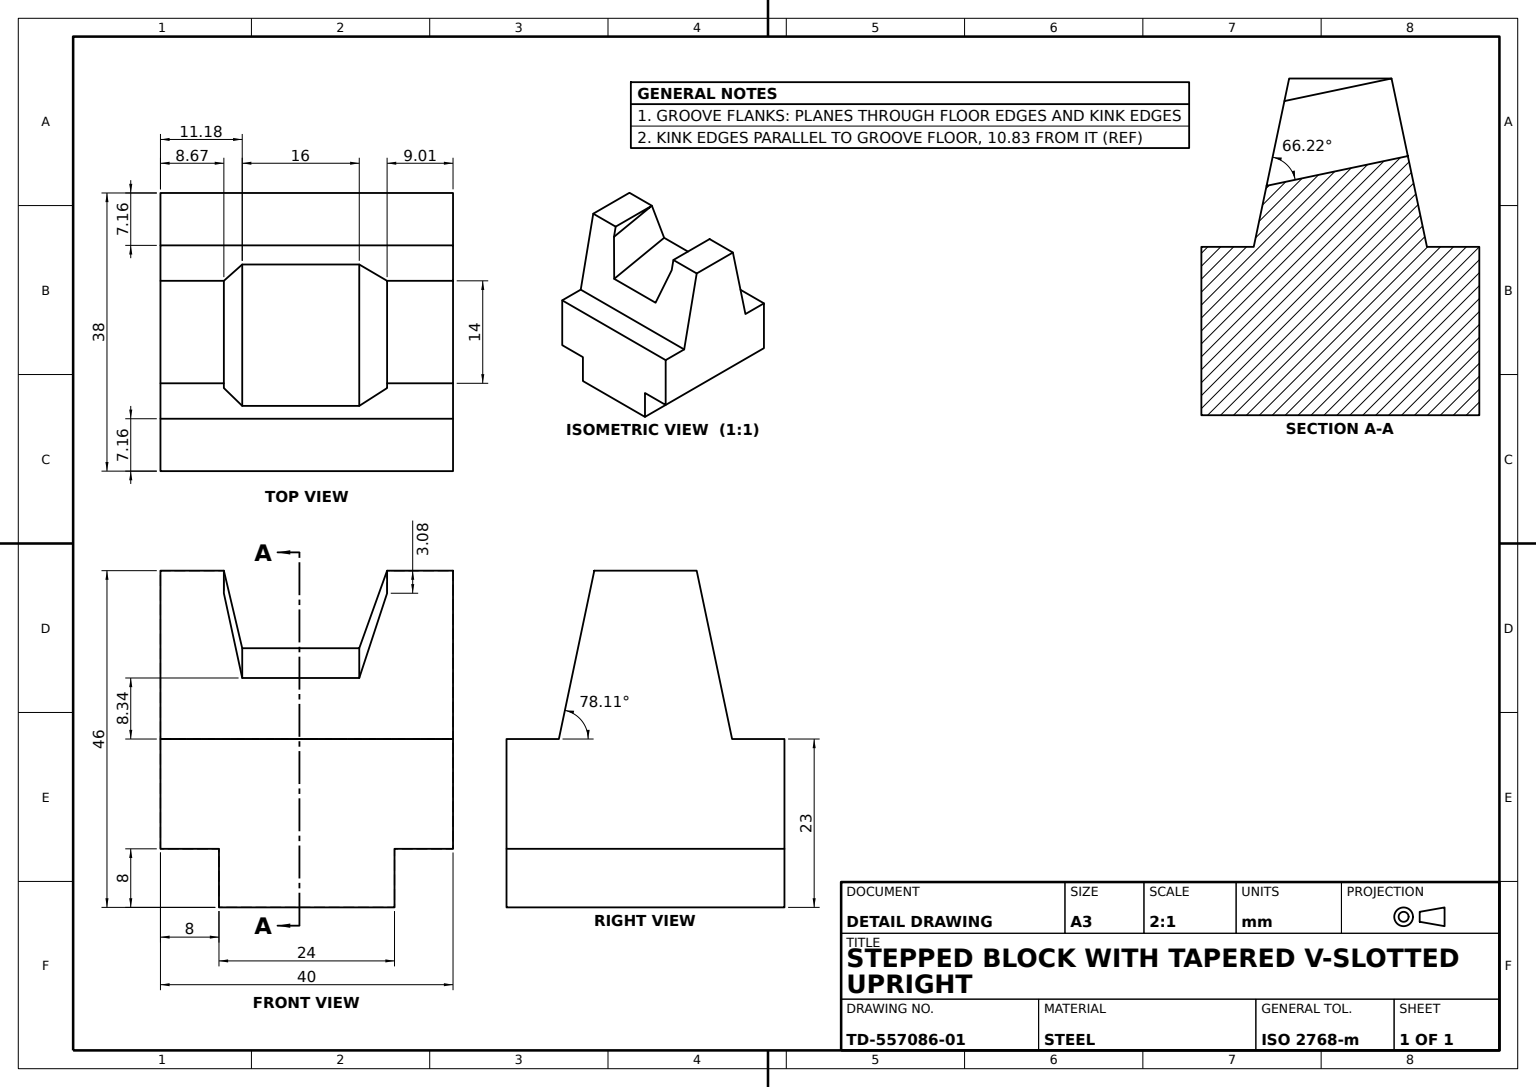
from build123d import *

# Parameters (mm, degrees)
BASE_PROFILE_SKETCH_W  = 40
BASE_PROFILE_SKETCH_H  = 46
BASE_BLOCK_DEPTH       = 38
BOTTOM_STEP_SKETCH_W   = 8
BOTTOM_STEP_SKETCH_H   = 8
BOTTOM_STEP_CUT_DEPTH  = 49.713447835
CORNER_NOTCH_SKETCH_W  = 8
CORNER_NOTCH_SKETCH_H  = 8
CORNER_NOTCH_8X8_DEPTH = 49.713447835
V_GROOVE_CUT_DEPTH     = 46
SLOT_CUT_8X8_DEPTH     = 46
SIDE_TRIM_SKETCH_W     = 22.317279544
SIDE_TRIM_SKETCH_H     = 4.669832792
SIDE_TRIM_CUT_DEPTH    = 46


with BuildPart() as part:
    # Base Profile Sketch → Base Block (new body)
    with BuildSketch(Plane.XY):
        Rectangle(BASE_PROFILE_SKETCH_W, BASE_PROFILE_SKETCH_H)
    extrude(amount=BASE_BLOCK_DEPTH)

    # Bottom Step Sketch → Bottom Step Cut (cut, through all)
    with BuildSketch(Plane.XY.offset(38)):
        with Locations((-16, -19)):
            Rectangle(BOTTOM_STEP_SKETCH_W, BOTTOM_STEP_SKETCH_H)
    extrude(amount=-BOTTOM_STEP_CUT_DEPTH, mode=Mode.SUBTRACT)

    # Corner Notch Sketch → Corner Notch 8x8 (cut, through all)
    with BuildSketch(Plane.XY.offset(38)):
        with Locations((16, -19)):
            Rectangle(CORNER_NOTCH_SKETCH_W, CORNER_NOTCH_SKETCH_H)
    extrude(amount=-CORNER_NOTCH_8X8_DEPTH, mode=Mode.SUBTRACT)

    # V-Groove Profile Sketch → V-Groove Cut (cut, symmetric)
    with BuildSketch(Plane(origin=(0, 0, 0), x_dir=(0, 0, -1), z_dir=(1, 0, 0))):
        Polygon((-38, 0), (-30.842105263, 0), (-26, 23), (-38, 23), align=None)
        Polygon((-12, 23), (-7.157894737, 0), (0, 0), (0, 23), align=None)
    extrude(amount=V_GROOVE_CUT_DEPTH, both=True, mode=Mode.SUBTRACT)

    # Slot Sketch → Slot Cut 8x8 (cut, symmetric)
    with BuildSketch(Plane(origin=(0, -1.442970822, 6.854111406), x_dir=(-1, 0, 0), z_dir=(0, 0.206010481049842, -0.9785497849867492))):
        Polygon((-7.180041029, 14.15108932), (0.819958971, 14.15108932), (8.819958971, 14.15108932), (11.331109989, 24.978770827), (-10.986169555, 24.978770827), align=None)
    extrude(amount=SLOT_CUT_8X8_DEPTH, both=True, mode=Mode.SUBTRACT)

    # Side Trim Sketch → Side Trim Cut (cut, symmetric)
    with BuildSketch(Plane(origin=(0, -1.442970822, 6.854111406), x_dir=(-1, 0, 0), z_dir=(0, 0.206010481049842, -0.9785497849867492))):
        with Locations((0.172470217, 27.313687223)):
            Rectangle(SIDE_TRIM_SKETCH_W, SIDE_TRIM_SKETCH_H)
    extrude(amount=SIDE_TRIM_CUT_DEPTH, both=True, mode=Mode.SUBTRACT)


solid = part.part
